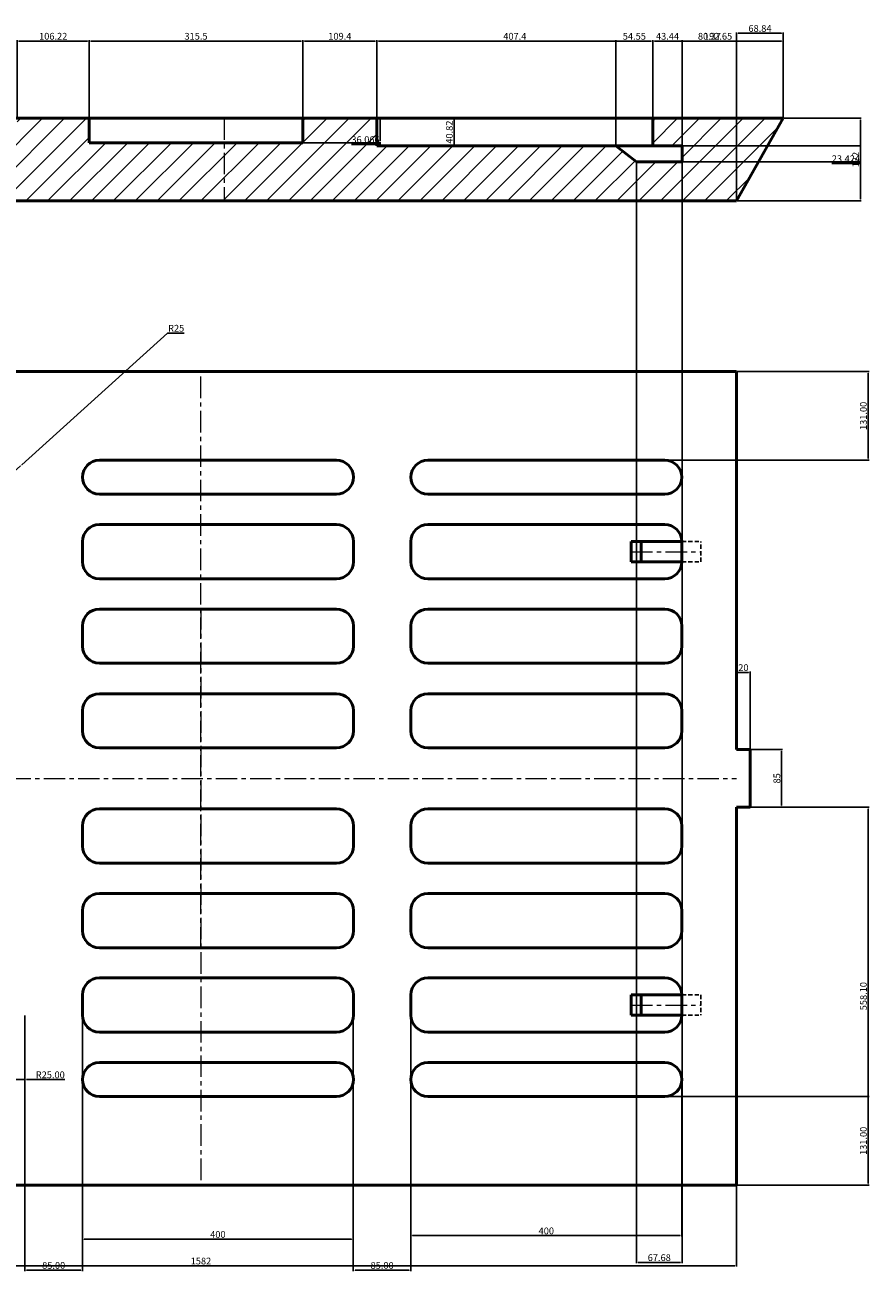
# Model space of a CAD drawing. Units: millimetres. Extents: x 1178 to 3717, y 924 to 2764.
# Tile 5 of 5: x 2471 to 3717, y 924 to 2764. Entities that reach past the tile are written whole.
import ezdxf

# ---------------------------------------------------------------- set-up
doc = ezdxf.new("R2010")
doc.units = ezdxf.units.MM
doc.linetypes.add('CENTER', pattern=[50.8, 31.75, -6.35, 6.35, -6.35])
doc.linetypes.add('HIDDEN', pattern=[9.525, 6.35, -3.175])
for name, color, linetype, lineweight in [('M-CNTR', 1, 'CENTER', 18), ('M-DIMS', 2, 'Continuous', 25), ('M-HATC', 8, 'Continuous', 18), ('M-HIDN', 6, 'HIDDEN', 25), ('M-OUTL', 7, 'Continuous', 50)]:
    doc.layers.add(name, color=color, linetype=linetype, lineweight=lineweight)
doc.styles.get("Standard").update_dxf_attribs({"font": 'arial.ttf'})
doc.dimstyles.new('ISO-25', dxfattribs={"dimtxt": 10, "dimasz": 2.5, "dimexe": 1.25, "dimexo": 0.625, "dimtad": 1, "dimtoh": 1, "dimdec": 0, "dimtxsty": 'Standard', "dimcen": 2.5, "dimadec": 0, "dimazin": 0, "dimtfac": 1, "dimtdec": 0, "dimtmove": 0, "dimatfit": 3, "dimfxl": 1, "dimarcsym": 0})

# ---------------------------------------------------------------- blocks, each defined once
blk = doc.blocks.new('*D1')
at = {"layer": 'Defpoints', "color": 0, "transparency": 16777216}
for p in [(1939.5, 1051), (3521.5, 1051), (3521.5, 932.1)]:
    blk.add_point(p, dxfattribs=at)
at = {"layer": 'M-DIMS', "color": 0, "lineweight": -2, "transparency": 16777216}
for p, q in [((1939.5, 1050.4), (1939.5, 930.9)), ((3521.5, 1050.4), (3521.5, 930.9)), ((1942, 932.1), (3519, 932.1))]:
    blk.add_line(p, q, dxfattribs=at)
at = {"layer": 'M-DIMS', "color": 0, "transparency": 16777216}
for points in [[(1942, 932.5), (1942, 931.7), (1939.5, 932.1)], [(3519, 932.5), (3519, 931.7), (3521.5, 932.1)]]:
    blk.add_solid(points, dxfattribs=at)
at = {"layer": 'M-DIMS', "color": 0, "transparency": 16777216, "insert": (2730.5, 937.8), "char_height": 10, "attachment_point": 5}
blk.add_mtext('1582', dxfattribs=at)
blk = doc.blocks.new('*D4')
at = {"layer": 'Defpoints', "color": 0, "transparency": 16777216}
for p in [(2555.5, 1207), (2955.5, 1207), (2955.5, 971.2)]:
    blk.add_point(p, dxfattribs=at)
at = {"layer": 'M-DIMS', "color": 0, "lineweight": -2, "transparency": 16777216}
for p, q in [((2555.5, 1206.4), (2555.5, 970)), ((2955.5, 1206.4), (2955.5, 970)), ((2558, 971.2), (2953, 971.2))]:
    blk.add_line(p, q, dxfattribs=at)
at = {"layer": 'M-DIMS', "color": 0, "transparency": 16777216}
for points in [[(2558, 971.7), (2558, 970.8), (2555.5, 971.2)], [(2953, 971.7), (2953, 970.8), (2955.5, 971.2)]]:
    blk.add_solid(points, dxfattribs=at)
at = {"layer": 'M-DIMS', "color": 0, "transparency": 16777216, "insert": (2755.5, 977), "char_height": 10, "attachment_point": 5}
blk.add_mtext('400', dxfattribs=at)
blk = doc.blocks.new('*D5')
at = {"layer": 'Defpoints', "color": 0, "transparency": 16777216}
for p in [(3040.5, 1207), (3440.5, 1207), (3440.5, 976.6)]:
    blk.add_point(p, dxfattribs=at)
at = {"layer": 'M-DIMS', "color": 0, "lineweight": -2, "transparency": 16777216}
for p, q in [((3040.5, 1206.4), (3040.5, 975.4)), ((3440.5, 1206.4), (3440.5, 975.4)), ((3043, 976.6), (3438, 976.6))]:
    blk.add_line(p, q, dxfattribs=at)
at = {"layer": 'M-DIMS', "color": 0, "transparency": 16777216}
for points in [[(3043, 977), (3043, 976.2), (3040.5, 976.6)], [(3438, 977), (3438, 976.2), (3440.5, 976.6)]]:
    blk.add_solid(points, dxfattribs=at)
at = {"layer": 'M-DIMS', "color": 0, "transparency": 16777216, "insert": (3240.5, 982.3), "char_height": 10, "attachment_point": 5}
blk.add_mtext('400', dxfattribs=at)
blk = doc.blocks.new('*D22')
at = {"layer": 'Defpoints', "color": 0, "transparency": 16777216}
for p in [(3541.5, 1694.1), (3541.5, 1609.1), (3587.9, 1609.1)]:
    blk.add_point(p, dxfattribs=at)
at = {"layer": 'M-DIMS', "color": 0, "lineweight": -2, "transparency": 16777216}
for p, q in [((3542.2, 1694.1), (3589.2, 1694.1)), ((3587.9, 1691.6), (3587.9, 1611.6)), ((3542.2, 1609.1), (3589.2, 1609.1))]:
    blk.add_line(p, q, dxfattribs=at)
at = {"layer": 'M-DIMS', "color": 0, "transparency": 16777216}
for points in [[(3587.5, 1691.6), (3588.3, 1691.6), (3587.9, 1694.1)], [(3587.5, 1611.6), (3588.3, 1611.6), (3587.9, 1609.1)]]:
    blk.add_solid(points, dxfattribs=at)
at = {"layer": 'M-DIMS', "color": 0, "transparency": 16777216, "insert": (3582.2, 1651.6), "char_height": 10, "attachment_point": 5, "rotation": 90}
blk.add_mtext('85', dxfattribs=at)
blk = doc.blocks.new('*D23')
at = {"layer": 'Defpoints', "color": 0, "transparency": 16777216}
for p in [(2464.1, 2113), (2445.5, 2096.2)]:
    blk.add_point(p, dxfattribs=at)
at = {"layer": 'M-DIMS', "color": 0, "lineweight": -2, "transparency": 16777216}
for p, q in [((2681.3, 2309), (2466, 2114.6)), ((2705.9, 2309), (2681.3, 2309)), ((2445.5, 2096.2), (2464.1, 2113))]:
    blk.add_line(p, q, dxfattribs=at)
at = {"layer": 'M-DIMS', "color": 0, "transparency": 16777216}
blk.add_solid([(2465.7, 2115), (2466.2, 2114.3), (2464.1, 2113)], dxfattribs=at)
at = {"layer": 'M-DIMS', "color": 0, "transparency": 16777216, "insert": (2693.9, 2314.8), "char_height": 10, "attachment_point": 5}
blk.add_mtext('R25', dxfattribs=at)
blk = doc.blocks.new('SLOT-400X80')
for p, q in [((375, 80), (25, 80)), ((0, 55), (0, 25)), ((400, 25), (400, 55)), ((25, 0), (375, 0))]:
    blk.add_line(p, q)
for centre, start, end in [((25, 55), 90, 180), ((375, 55), 0, 90), ((25, 25), 180, 270), ((375, 25), 270, 0)]:
    blk.add_arc(centre, 25, start, end)
blk = doc.blocks.new('SLOT-400X50')
for p, q in [((375, 50), (25, 50)), ((25, 0), (375, 0))]:
    blk.add_line(p, q)
for centre, start, end in [((25, 25), 90, 270), ((375, 25), 270, 90)]:
    blk.add_arc(centre, 25, start, end)
blk = doc.blocks.new('*D31')
at = {"layer": 'Defpoints', "color": 0, "transparency": 16777216}
for p in [(2565.4, 2740), (2459.2, 2626), (2565.4, 2626)]:
    blk.add_point(p, dxfattribs=at)
at = {"layer": 'M-DIMS', "color": 0, "lineweight": -2, "transparency": 16777216}
for p, q in [((2459.2, 2626.7), (2459.2, 2741.3)), ((2565.4, 2626.7), (2565.4, 2741.3)), ((2461.7, 2740), (2562.9, 2740))]:
    blk.add_line(p, q, dxfattribs=at)
at = {"layer": 'M-DIMS', "color": 0, "transparency": 16777216}
for points in [[(2461.7, 2740.5), (2461.7, 2739.6), (2459.2, 2740)], [(2562.9, 2740.5), (2562.9, 2739.6), (2565.4, 2740)]]:
    blk.add_solid(points, dxfattribs=at)
at = {"layer": 'M-DIMS', "color": 0, "transparency": 16777216, "insert": (2512.3, 2745.8), "char_height": 10, "attachment_point": 5}
blk.add_mtext('106.22', dxfattribs=at)
blk = doc.blocks.new('*D32')
at = {"layer": 'Defpoints', "color": 0, "transparency": 16777216}
for p in [(2880.9, 2740), (2565.4, 2626), (2880.9, 2626)]:
    blk.add_point(p, dxfattribs=at)
at = {"layer": 'M-DIMS', "color": 0, "lineweight": -2, "transparency": 16777216}
for p, q in [((2565.4, 2626.7), (2565.4, 2741.3)), ((2880.9, 2626.7), (2880.9, 2741.3)), ((2567.9, 2740), (2878.4, 2740))]:
    blk.add_line(p, q, dxfattribs=at)
at = {"layer": 'M-DIMS', "color": 0, "transparency": 16777216}
for points in [[(2567.9, 2740.5), (2567.9, 2739.6), (2565.4, 2740)], [(2878.4, 2740.5), (2878.4, 2739.6), (2880.9, 2740)]]:
    blk.add_solid(points, dxfattribs=at)
at = {"layer": 'M-DIMS', "color": 0, "transparency": 16777216, "insert": (2723.2, 2745.8), "char_height": 10, "attachment_point": 5}
blk.add_mtext('315.5', dxfattribs=at)
blk = doc.blocks.new('*D33')
at = {"layer": 'Defpoints', "color": 0, "transparency": 16777216}
for p in [(2990.3, 2740), (2880.9, 2626), (2990.3, 2626)]:
    blk.add_point(p, dxfattribs=at)
at = {"layer": 'M-DIMS', "color": 0, "lineweight": -2, "transparency": 16777216}
for p, q in [((2880.9, 2626.7), (2880.9, 2741.3)), ((2990.3, 2626.7), (2990.3, 2741.3)), ((2883.4, 2740), (2987.8, 2740))]:
    blk.add_line(p, q, dxfattribs=at)
at = {"layer": 'M-DIMS', "color": 0, "transparency": 16777216}
for points in [[(2883.4, 2740.5), (2883.4, 2739.6), (2880.9, 2740)], [(2987.8, 2740.5), (2987.8, 2739.6), (2990.3, 2740)]]:
    blk.add_solid(points, dxfattribs=at)
at = {"layer": 'M-DIMS', "color": 0, "transparency": 16777216, "insert": (2935.6, 2745.8), "char_height": 10, "attachment_point": 5}
blk.add_mtext('109.4', dxfattribs=at)
blk = doc.blocks.new('*D34')
at = {"layer": 'Defpoints', "color": 0, "transparency": 16777216}
for p in [(3397.7, 2740), (2990.3, 2626), (3397.7, 2626)]:
    blk.add_point(p, dxfattribs=at)
at = {"layer": 'M-DIMS', "color": 0, "lineweight": -2, "transparency": 16777216}
for p, q in [((2990.3, 2626.7), (2990.3, 2741.3)), ((3397.7, 2626.7), (3397.7, 2741.3)), ((2992.8, 2740), (3395.2, 2740))]:
    blk.add_line(p, q, dxfattribs=at)
at = {"layer": 'M-DIMS', "color": 0, "transparency": 16777216}
for points in [[(2992.8, 2740.5), (2992.8, 2739.6), (2990.3, 2740)], [(3395.2, 2740.5), (3395.2, 2739.6), (3397.7, 2740)]]:
    blk.add_solid(points, dxfattribs=at)
at = {"layer": 'M-DIMS', "color": 0, "transparency": 16777216, "insert": (3194, 2745.8), "char_height": 10, "attachment_point": 5}
blk.add_mtext('407.4', dxfattribs=at)
blk = doc.blocks.new('*D35')
at = {"layer": 'Defpoints', "color": 0, "transparency": 16777216}
for p in [(3590.4, 2740), (3397.7, 2626), (3590.4, 2626)]:
    blk.add_point(p, dxfattribs=at)
at = {"layer": 'M-DIMS', "color": 0, "lineweight": -2, "transparency": 16777216}
for p, q in [((3397.7, 2626.7), (3397.7, 2741.3)), ((3590.4, 2626.7), (3590.4, 2741.3)), ((3400.2, 2740), (3587.9, 2740))]:
    blk.add_line(p, q, dxfattribs=at)
at = {"layer": 'M-DIMS', "color": 0, "transparency": 16777216}
for points in [[(3400.2, 2740.5), (3400.2, 2739.6), (3397.7, 2740)], [(3587.9, 2740.5), (3587.9, 2739.6), (3590.4, 2740)]]:
    blk.add_solid(points, dxfattribs=at)
at = {"layer": 'M-DIMS', "color": 0, "transparency": 16777216, "insert": (3494.1, 2745.8), "char_height": 10, "attachment_point": 5}
blk.add_mtext('192.65', dxfattribs=at)
blk = doc.blocks.new('*D36')
at = {"layer": 'Defpoints', "color": 0, "transparency": 16777216}
for p in [(3590.4, 2626), (3521.5, 2504), (3704.4, 2504)]:
    blk.add_point(p, dxfattribs=at)
at = {"layer": 'M-DIMS', "color": 0, "lineweight": -2, "transparency": 16777216}
for p, q in [((3591, 2626), (3705.6, 2626)), ((3704.4, 2623.5), (3704.4, 2506.5)), ((3522.2, 2504), (3705.6, 2504))]:
    blk.add_line(p, q, dxfattribs=at)
at = {"layer": 'M-DIMS', "color": 0, "transparency": 16777216}
for points in [[(3704, 2623.5), (3704.8, 2623.5), (3704.4, 2626)], [(3704, 2506.5), (3704.8, 2506.5), (3704.4, 2504)]]:
    blk.add_solid(points, dxfattribs=at)
at = {"layer": 'M-DIMS', "color": 0, "transparency": 16777216, "insert": (3698.7, 2565), "char_height": 10, "attachment_point": 5, "rotation": 90}
blk.add_mtext('122', dxfattribs=at)
blk = doc.blocks.new('*D37')
at = {"layer": 'Defpoints', "color": 0, "transparency": 16777216}
for p in [(2880.9, 2626), (2880.9, 2590), (2994.9, 2590)]:
    blk.add_point(p, dxfattribs=at)
at = {"layer": 'M-DIMS', "color": 0, "lineweight": -2, "transparency": 16777216}
for p, q in [((2881.5, 2626), (2996.1, 2626)), ((2994.9, 2623.5), (2994.9, 2592.5)), ((2881.5, 2590), (2996.1, 2590)), ((2994.9, 2587.5), (2952.8, 2587.5)), ((2994.9, 2590), (2994.9, 2587.5))]:
    blk.add_line(p, q, dxfattribs=at)
at = {"layer": 'M-DIMS', "color": 0, "transparency": 16777216}
for points in [[(2994.5, 2623.5), (2995.3, 2623.5), (2994.9, 2626)], [(2994.5, 2592.5), (2995.3, 2592.5), (2994.9, 2590)]]:
    blk.add_solid(points, dxfattribs=at)
at = {"layer": 'M-DIMS', "color": 0, "transparency": 16777216, "insert": (2973.5, 2593.2), "char_height": 10, "attachment_point": 5}
blk.add_mtext('36.066', dxfattribs=at)
blk = doc.blocks.new('*D38')
at = {"layer": 'Defpoints', "color": 0, "transparency": 16777216}
for p in [(2990.3, 2626), (2990.3, 2585.2), (3104.3, 2585.2)]:
    blk.add_point(p, dxfattribs=at)
at = {"layer": 'M-DIMS', "color": 0, "lineweight": -2, "transparency": 16777216}
for p, q in [((2990.9, 2626), (3105.5, 2626)), ((3104.3, 2623.5), (3104.3, 2587.7)), ((2990.9, 2585.2), (3105.5, 2585.2))]:
    blk.add_line(p, q, dxfattribs=at)
at = {"layer": 'M-DIMS', "color": 0, "transparency": 16777216}
for points in [[(3103.9, 2623.5), (3104.7, 2623.5), (3104.3, 2626)], [(3103.9, 2587.7), (3104.7, 2587.7), (3104.3, 2585.2)]]:
    blk.add_solid(points, dxfattribs=at)
at = {"layer": 'M-DIMS', "color": 0, "transparency": 16777216, "insert": (3098.6, 2605.6), "char_height": 10, "attachment_point": 5, "rotation": 90}
blk.add_mtext('40.82', dxfattribs=at)
blk = doc.blocks.new('*D44')
at = {"layer": 'Defpoints', "color": 0, "transparency": 16777216}
for p in [(3397.7, 2740), (3343.2, 2585.2), (3397.7, 2585.2)]:
    blk.add_point(p, dxfattribs=at)
at = {"layer": 'M-DIMS', "color": 0, "lineweight": -2, "transparency": 16777216}
for p, q in [((3343.2, 2585.8), (3343.2, 2741.3)), ((3397.7, 2585.8), (3397.7, 2741.3)), ((3345.7, 2740), (3395.2, 2740))]:
    blk.add_line(p, q, dxfattribs=at)
at = {"layer": 'M-DIMS', "color": 0, "transparency": 16777216}
for points in [[(3345.7, 2740.5), (3345.7, 2739.6), (3343.2, 2740)], [(3395.2, 2740.5), (3395.2, 2739.6), (3397.7, 2740)]]:
    blk.add_solid(points, dxfattribs=at)
at = {"layer": 'M-DIMS', "color": 0, "transparency": 16777216, "insert": (3370.5, 2745.8), "char_height": 10, "attachment_point": 5}
blk.add_mtext('54.55', dxfattribs=at)
blk = doc.blocks.new('*D45')
at = {"layer": 'Defpoints', "color": 0, "transparency": 16777216}
for p in [(3441.2, 2740), (3397.7, 2585.2), (3441.2, 2585.2)]:
    blk.add_point(p, dxfattribs=at)
at = {"layer": 'M-DIMS', "color": 0, "lineweight": -2, "transparency": 16777216}
for p, q in [((3397.7, 2585.8), (3397.7, 2741.3)), ((3441.2, 2585.8), (3441.2, 2741.3)), ((3400.2, 2740), (3438.7, 2740))]:
    blk.add_line(p, q, dxfattribs=at)
at = {"layer": 'M-DIMS', "color": 0, "transparency": 16777216}
for points in [[(3400.2, 2740.5), (3400.2, 2739.6), (3397.7, 2740)], [(3438.7, 2740.5), (3438.7, 2739.6), (3441.2, 2740)]]:
    blk.add_solid(points, dxfattribs=at)
at = {"layer": 'M-DIMS', "color": 0, "transparency": 16777216, "insert": (3419.5, 2745.8), "char_height": 10, "attachment_point": 5}
blk.add_mtext('43.44', dxfattribs=at)
blk = doc.blocks.new('*D46')
at = {"layer": 'Defpoints', "color": 0, "transparency": 16777216}
for p in [(3521.5, 2740), (3441.2, 2585.2), (3521.5, 2504)]:
    blk.add_point(p, dxfattribs=at)
at = {"layer": 'M-DIMS', "color": 0, "lineweight": -2, "transparency": 16777216}
for p, q in [((3441.2, 2585.8), (3441.2, 2741.3)), ((3521.5, 2504.7), (3521.5, 2741.3)), ((3443.7, 2740), (3519, 2740))]:
    blk.add_line(p, q, dxfattribs=at)
at = {"layer": 'M-DIMS', "color": 0, "transparency": 16777216}
for points in [[(3443.7, 2740.5), (3443.7, 2739.6), (3441.2, 2740)], [(3519, 2740.5), (3519, 2739.6), (3521.5, 2740)]]:
    blk.add_solid(points, dxfattribs=at)
at = {"layer": 'M-DIMS', "color": 0, "transparency": 16777216, "insert": (3481.4, 2745.8), "char_height": 10, "attachment_point": 5}
blk.add_mtext('80.37', dxfattribs=at)
blk = doc.blocks.new('*D47')
at = {"layer": 'Defpoints', "color": 0, "transparency": 16777216}
for p in [(3373.5, 2561.8), (3441.2, 2561.8), (3441.2, 937)]:
    blk.add_point(p, dxfattribs=at)
at = {"layer": 'M-DIMS', "color": 0, "lineweight": -2, "transparency": 16777216}
for p, q in [((3373.5, 2561.2), (3373.5, 935.8)), ((3441.2, 2561.2), (3441.2, 935.8)), ((3376, 937), (3438.7, 937))]:
    blk.add_line(p, q, dxfattribs=at)
at = {"layer": 'M-DIMS', "color": 0, "transparency": 16777216}
for points in [[(3376, 937.4), (3376, 936.6), (3373.5, 937)], [(3438.7, 937.4), (3438.7, 936.6), (3441.2, 937)]]:
    blk.add_solid(points, dxfattribs=at)
at = {"layer": 'M-DIMS', "color": 0, "transparency": 16777216, "insert": (3407.3, 942.8), "char_height": 10, "attachment_point": 5}
blk.add_mtext('67.68', dxfattribs=at)
blk = doc.blocks.new('*D48')
at = {"layer": 'Defpoints', "color": 0, "transparency": 16777216}
for p in [(3441.2, 2585.2), (3441.2, 2561.8), (3704.4, 2561.8)]:
    blk.add_point(p, dxfattribs=at)
at = {"layer": 'M-DIMS', "color": 0, "lineweight": -2, "transparency": 16777216}
for p, q in [((3441.8, 2585.2), (3705.6, 2585.2)), ((3704.4, 2582.7), (3704.4, 2564.3)), ((3441.8, 2561.8), (3705.6, 2561.8)), ((3704.4, 2559.3), (3662.1, 2559.3)), ((3704.4, 2561.8), (3704.4, 2559.3))]:
    blk.add_line(p, q, dxfattribs=at)
at = {"layer": 'M-DIMS', "color": 0, "transparency": 16777216}
for points in [[(3704, 2582.7), (3704.8, 2582.7), (3704.4, 2585.2)], [(3704, 2564.3), (3704.8, 2564.3), (3704.4, 2561.8)]]:
    blk.add_solid(points, dxfattribs=at)
at = {"layer": 'M-DIMS', "color": 0, "transparency": 16777216, "insert": (3682.9, 2565), "char_height": 10, "attachment_point": 5}
blk.add_mtext('23.424', dxfattribs=at)
blk = doc.blocks.new('*D57')
at = {"layer": 'Defpoints', "color": 0, "transparency": 16777216}
for p in [(3541.5, 1808.1), (3521.5, 1694.1), (3541.5, 1694.1)]:
    blk.add_point(p, dxfattribs=at)
at = {"layer": 'M-DIMS', "color": 0, "lineweight": -2, "transparency": 16777216}
for p, q in [((3521.5, 1694.7), (3521.5, 1809.4)), ((3524, 1808.1), (3539, 1808.1)), ((3541.5, 1694.7), (3541.5, 1809.4))]:
    blk.add_line(p, q, dxfattribs=at)
at = {"layer": 'M-DIMS', "color": 0, "transparency": 16777216}
for points in [[(3524, 1808.5), (3524, 1807.7), (3521.5, 1808.1)], [(3539, 1808.5), (3539, 1807.7), (3541.5, 1808.1)]]:
    blk.add_solid(points, dxfattribs=at)
at = {"layer": 'M-DIMS', "color": 0, "transparency": 16777216, "insert": (3531.5, 1813.8), "char_height": 10, "attachment_point": 5}
blk.add_mtext('20', dxfattribs=at)
blk = doc.blocks.new('*D65')
at = {"layer": 'Defpoints', "color": 0, "transparency": 16777216}
for p in [(3521.5, 2751.5), (3590.4, 2626), (3521.5, 2504)]:
    blk.add_point(p, dxfattribs=at)
at = {"layer": 'M-DIMS', "color": 0, "lineweight": -2, "transparency": 16777216}
for p, q in [((3521.5, 2504.7), (3521.5, 2752.8)), ((3587.9, 2751.5), (3524, 2751.5)), ((3590.4, 2626.7), (3590.4, 2752.8))]:
    blk.add_line(p, q, dxfattribs=at)
at = {"layer": 'M-DIMS', "color": 0, "transparency": 16777216}
for points in [[(3524, 2752), (3524, 2751.1), (3521.5, 2751.5)], [(3587.9, 2752), (3587.9, 2751.1), (3590.4, 2751.5)]]:
    blk.add_solid(points, dxfattribs=at)
at = {"layer": 'M-DIMS', "color": 0, "transparency": 16777216, "insert": (3556, 2757.3), "char_height": 10, "attachment_point": 5}
blk.add_mtext('68.84', dxfattribs=at)
blk = doc.blocks.new('*D66')
at = {"layer": 'Defpoints', "color": 0, "transparency": 16777216}
for p in [(2470.5, 1302), (2555.5, 1302), (2555.5, 925.5)]:
    blk.add_point(p, dxfattribs=at)
at = {"layer": 'M-DIMS', "color": 0, "lineweight": -2, "transparency": 16777216}
for p, q in [((2470.5, 1301.4), (2470.5, 924.3)), ((2555.5, 1301.4), (2555.5, 924.3)), ((2473, 925.5), (2553, 925.5))]:
    blk.add_line(p, q, dxfattribs=at)
at = {"layer": 'M-DIMS', "color": 0, "transparency": 16777216}
for points in [[(2473, 925.9), (2473, 925.1), (2470.5, 925.5)], [(2553, 925.9), (2553, 925.1), (2555.5, 925.5)]]:
    blk.add_solid(points, dxfattribs=at)
at = {"layer": 'M-DIMS', "color": 0, "transparency": 16777216, "insert": (2513, 931.3), "char_height": 10, "attachment_point": 5}
blk.add_mtext('85.00', dxfattribs=at)
blk = doc.blocks.new('*D67')
at = {"layer": 'Defpoints', "color": 0, "transparency": 16777216}
for p in [(2955.5, 1302), (3040.5, 1302), (3040.5, 925.5)]:
    blk.add_point(p, dxfattribs=at)
at = {"layer": 'M-DIMS', "color": 0, "lineweight": -2, "transparency": 16777216}
for p, q in [((2955.5, 1301.4), (2955.5, 924.3)), ((3040.5, 1301.4), (3040.5, 924.3)), ((2958, 925.5), (3038, 925.5))]:
    blk.add_line(p, q, dxfattribs=at)
at = {"layer": 'M-DIMS', "color": 0, "transparency": 16777216}
for points in [[(2958, 925.9), (2958, 925.1), (2955.5, 925.5)], [(3038, 925.9), (3038, 925.1), (3040.5, 925.5)]]:
    blk.add_solid(points, dxfattribs=at)
at = {"layer": 'M-DIMS', "color": 0, "transparency": 16777216, "insert": (2998, 931.3), "char_height": 10, "attachment_point": 5}
blk.add_mtext('85.00', dxfattribs=at)
blk = doc.blocks.new('*D68')
at = {"layer": 'Defpoints', "color": 0, "transparency": 16777216}
for p in [(3521.5, 2252.2), (3715.9, 2252.2), (3415.5, 2121.2)]:
    blk.add_point(p, dxfattribs=at)
at = {"layer": 'M-DIMS', "color": 0, "lineweight": -2, "transparency": 16777216}
for p, q in [((3522.2, 2252.2), (3717.1, 2252.2)), ((3715.9, 2123.7), (3715.9, 2249.7)), ((3416.2, 2121.2), (3717.1, 2121.2))]:
    blk.add_line(p, q, dxfattribs=at)
at = {"layer": 'M-DIMS', "color": 0, "transparency": 16777216}
for points in [[(3715.5, 2249.7), (3716.3, 2249.7), (3715.9, 2252.2)], [(3715.5, 2123.7), (3716.3, 2123.7), (3715.9, 2121.2)]]:
    blk.add_solid(points, dxfattribs=at)
at = {"layer": 'M-DIMS', "color": 0, "transparency": 16777216, "insert": (3710.1, 2186.7), "char_height": 10, "attachment_point": 5, "rotation": 90}
blk.add_mtext('131.00', dxfattribs=at)
blk = doc.blocks.new('*D69')
at = {"layer": 'Defpoints', "color": 0, "transparency": 16777216}
for p in [(3415.5, 1182), (3521.5, 1051), (3715.9, 1051)]:
    blk.add_point(p, dxfattribs=at)
at = {"layer": 'M-DIMS', "color": 0, "lineweight": -2, "transparency": 16777216}
for p, q in [((3416.2, 1182), (3717.1, 1182)), ((3715.9, 1179.5), (3715.9, 1053.5)), ((3522.2, 1051), (3717.1, 1051))]:
    blk.add_line(p, q, dxfattribs=at)
at = {"layer": 'M-DIMS', "color": 0, "transparency": 16777216}
for points in [[(3715.5, 1179.5), (3716.3, 1179.5), (3715.9, 1182)], [(3715.5, 1053.5), (3716.3, 1053.5), (3715.9, 1051)]]:
    blk.add_solid(points, dxfattribs=at)
at = {"layer": 'M-DIMS', "color": 0, "transparency": 16777216, "insert": (3710.1, 1116.5), "char_height": 10, "attachment_point": 5, "rotation": 90}
blk.add_mtext('131.00', dxfattribs=at)
blk = doc.blocks.new('*D71')
at = {"layer": 'Defpoints', "color": 0, "transparency": 16777216}
for p in [(3541.5, 1609.1), (3715.9, 1609.1), (3521.5, 1051)]:
    blk.add_point(p, dxfattribs=at)
at = {"layer": 'M-DIMS', "color": 0, "lineweight": -2, "transparency": 16777216}
for p, q in [((3542.2, 1609.1), (3717.1, 1609.1)), ((3715.9, 1053.5), (3715.9, 1606.6)), ((3522.2, 1051), (3717.1, 1051))]:
    blk.add_line(p, q, dxfattribs=at)
at = {"layer": 'M-DIMS', "color": 0, "transparency": 16777216}
for points in [[(3715.5, 1606.6), (3716.3, 1606.6), (3715.9, 1609.1)], [(3715.5, 1053.5), (3716.3, 1053.5), (3715.9, 1051)]]:
    blk.add_solid(points, dxfattribs=at)
at = {"layer": 'M-DIMS', "color": 0, "transparency": 16777216, "insert": (3710.1, 1330.1), "char_height": 10, "attachment_point": 5, "rotation": 90}
blk.add_mtext('558.10', dxfattribs=at)
blk = doc.blocks.new('*D99')
at = {"layer": 'Defpoints', "color": 0, "transparency": 16777216}
for p in [(2445.5, 1207), (2470.5, 1207)]:
    blk.add_point(p, dxfattribs=at)
at = {"layer": 'M-DIMS', "color": 0, "lineweight": -2, "transparency": 16777216}
for p, q in [((2445.5, 1207), (2470.5, 1207)), ((2485.8, 1207), (2473, 1207)), ((2529.7, 1207), (2485.8, 1207))]:
    blk.add_line(p, q, dxfattribs=at)
at = {"layer": 'M-DIMS', "color": 0, "transparency": 16777216}
blk.add_solid([(2473, 1207.4), (2473, 1206.6), (2470.5, 1207)], dxfattribs=at)
at = {"layer": 'M-DIMS', "color": 0, "transparency": 16777216, "insert": (2508, 1212.7), "char_height": 10, "attachment_point": 5}
blk.add_mtext('R25.00', dxfattribs=at)

msp = doc.modelspace()

# ---------------------------------------------------------------- hatches: boundary and pattern name
at = {"layer": 'M-HATC'}
h = msp.add_hatch(dxfattribs=at)
h.set_pattern_fill('ANSI31', color=256, scale=7.2)
h.paths.add_polyline_path([(2053.3369, 2597.896), (2086.6296, 2597.896), (2086.6296, 2626.0416), (1939.5398, 2626.0416), (1878.7536, 2626.0416), (1939.5398, 2504.0416), (2764.9597, 2504.0416), (2764.9597, 2589.9761), (2565.4108, 2589.9761), (2565.4108, 2626.0416), (2459.1911, 2626.0416), (2459.1911, 2597.896), (2161.8062, 2597.896), (2107.2394, 2567.8003), (2053.3369, 2567.8003)])
h.paths.add_polyline_path([(3590.3795, 2626.0416), (3397.729, 2626.0416), (3397.729, 2585.2241), (3441.1717, 2585.2241), (3441.1717, 2561.8005), (3373.4902, 2561.8005), (3343.1801, 2585.2241), (2990.2894, 2585.2241), (2990.2894, 2626.0416), (2880.899, 2626.0416), (2880.899, 2589.9761), (2764.9597, 2589.9761), (2764.9597, 2504.0416), (3521.5398, 2504.0416)])

# ---------------------------------------------------------------- linework, layer by layer
at = {"layer": 'M-CNTR'}
for p, q in [((2764.9597, 2626.0416), (2764.9597, 2504.0416)), ((2730.5398, 1400.2134), (2730.5398, 2252.2134)), ((3365.7289, 1986.2134), (3468.7539, 1986.2134)), ((2730.5398, 1903.0224), (2730.5398, 1051.0224)), ((1939.5398, 1651.6179), (3521.5398, 1651.6179)), ((3365.7289, 1317.0224), (3468.7539, 1317.0224))]:
    msp.add_line(p, q, dxfattribs=at)
at = {"layer": 'M-HIDN'}
for p, q in [((3440.5398, 2001.2134), (3468.7539, 2001.2134)), ((3468.7539, 1971.2134), (3468.7539, 2001.2134)), ((3440.5398, 1971.2134), (3468.7539, 1971.2134)), ((3440.5398, 1332.0224), (3468.7539, 1332.0224)), ((3468.7539, 1332.0224), (3468.7539, 1302.0224)), ((3440.5398, 1302.0224), (3468.7539, 1302.0224))]:
    msp.add_line(p, q, dxfattribs=at)
at = {"layer": 'M-OUTL'}
for p, q in [((1939.5398, 2626.0416), (3590.3795, 2626.0416)), ((2565.4108, 2626.0416), (2565.4108, 2589.9761)), ((2880.899, 2589.9761), (2880.899, 2626.0416)), ((2990.2894, 2626.0416), (2990.2894, 2585.2241)), ((3397.729, 2585.2241), (3397.729, 2626.0416)), ((3590.3795, 2626.0416), (3521.5398, 2504.0416)), ((2565.4108, 2589.9761), (2880.899, 2589.9761)), ((2990.2894, 2585.2241), (3397.729, 2585.2241)), ((3373.4902, 2561.8005), (3343.1801, 2585.2241)), ((3397.729, 2585.2241), (3441.1717, 2585.2241)), ((3441.1717, 2585.2241), (3441.1717, 2561.8005)), ((3441.1717, 2561.8005), (3373.4902, 2561.8005)), ((3521.5398, 2504.0416), (1939.5398, 2504.0416)), ((2095.5398, 2252.2134), (3521.5398, 2252.2134)), ((3521.5398, 1903.0224), (3521.5398, 2252.2134)), ((3065.5398, 2026.2134), (3415.5398, 2026.2134)), ((3040.5398, 1971.2134), (3040.5398, 2001.2134)), ((3440.5398, 2001.2134), (3365.7289, 2001.2134)), ((3365.7289, 1971.2134), (3365.7289, 2001.2134)), ((3380.4882, 1971.2134), (3380.4882, 2001.2134)), ((3440.5398, 2001.2134), (3440.5398, 1971.2134)), ((3440.5398, 2001.2134), (3440.5398, 1971.2134)), ((3440.5398, 1971.2134), (3365.7289, 1971.2134)), ((3415.5398, 1946.2134), (3065.5398, 1946.2134)), ((3521.5398, 1694.1179), (3521.5398, 1903.0224)), ((3521.5398, 1694.1179), (3541.5398, 1694.1179)), ((3541.5398, 1694.1179), (3541.5398, 1609.1179)), ((3521.5398, 1051.0224), (3521.5398, 1609.1179)), ((3541.5398, 1609.1179), (3521.5398, 1609.1179)), ((3415.5398, 1357.0224), (3065.5398, 1357.0224)), ((3040.5398, 1332.0224), (3040.5398, 1302.0224)), ((3440.5398, 1332.0224), (3365.7289, 1332.0224)), ((3365.7289, 1332.0224), (3365.7289, 1302.0224)), ((3380.4882, 1332.0224), (3380.4882, 1302.0224)), ((3440.5398, 1302.0224), (3440.5398, 1332.0224)), ((3440.5398, 1302.0224), (3365.7289, 1302.0224)), ((3065.5398, 1277.0224), (3415.5398, 1277.0224)), ((1939.5398, 1051.0224), (3521.5398, 1051.0224))]:
    msp.add_line(p, q, dxfattribs=at)
for centre, start, end in [((3065.5398, 2001.2134), 90, 180), ((3415.5398, 2001.2134), 0, 90), ((3065.5398, 1971.2134), 180, 270), ((3415.5398, 1971.2134), 270, 0), ((3065.5398, 1332.0224), 90, 180), ((3415.5398, 1332.0224), 0, 90), ((3065.5398, 1302.0224), 180, 270), ((3415.5398, 1302.0224), 270, 0)]:
    msp.add_arc(centre, 25, start, end, dxfattribs=at)

# ---------------------------------------------------------------- block references
at = {"layer": 'M-OUTL', "rotation": 180}
for p in [(2955.5396, 2121.2139), (3440.5396, 2121.2139)]:
    msp.add_blockref('SLOT-400X50', p, dxfattribs=at)
at = {"layer": 'M-OUTL'}
for name, p in [('SLOT-400X80', (2555.54, 1946.213)), ('SLOT-400X80', (2555.54, 1821.6175)), ('SLOT-400X80', (3040.54, 1821.6175)), ('SLOT-400X80', (2555.54, 1696.6175)), ('SLOT-400X80', (3040.54, 1696.6175)), ('SLOT-400X80', (2555.54, 1526.6175)), ('SLOT-400X80', (3040.54, 1526.6175)), ('SLOT-400X80', (2555.54, 1401.6175)), ('SLOT-400X80', (3040.54, 1401.6175)), ('SLOT-400X80', (2555.54, 1277.022)), ('SLOT-400X50', (2555.54, 1182.022)), ('SLOT-400X50', (3040.54, 1182.022))]:
    msp.add_blockref(name, p, dxfattribs=at)

# ---------------------------------------------------------------- dimensions: what is measured, and where the dimension line sits
at = {"layer": 'M-DIMS'}
for base, p1, p2, override, picture, middle in [((3521.5398, 2751.5416), (3590.3795, 2626.0416), (3521.5398, 2504.0416), {"dimdec": 2, "dimlfac": 1, "dimrnd": 0, "dimzin": 0, "dimdsep": 46, "dimlunit": 2}, '*D65', (3555.9597, 2757.2723)), ((2565.4108, 2740.0416), (2459.1911, 2626.0416), (2565.4108, 2626.0416), {"dimdec": 2, "dimlfac": 1, "dimrnd": 0, "dimzin": 0, "dimdsep": 46, "dimlunit": 2}, '*D31', (2512.3009, 2745.7723)), ((2880.899, 2740.0416), (2565.4108, 2626.0416), (2880.899, 2626.0416), {"dimdec": 1, "dimlfac": 1, "dimrnd": 0, "dimzin": 0, "dimdsep": 46, "dimlunit": 2}, '*D32', (2723.1549, 2745.7757)), ((2990.2894, 2740.0416), (2880.899, 2626.0416), (2990.2894, 2626.0416), {"dimdec": 1, "dimlfac": 1, "dimrnd": 0, "dimzin": 0, "dimdsep": 46, "dimlunit": 2}, '*D33', (2935.5942, 2745.7723)), ((3397.729, 2740.0416), (2990.2894, 2626.0416), (3397.729, 2626.0416), {"dimdec": 1, "dimlfac": 1, "dimrnd": 0, "dimzin": 0, "dimdsep": 46, "dimlunit": 2}, '*D34', (3194.0092, 2745.7723)), ((3397.729, 2740.0416), (3343.1801, 2585.2241), (3397.729, 2585.2241), {"dimdec": 2, "dimlfac": 1, "dimrnd": 0, "dimzin": 0, "dimdsep": 46, "dimlunit": 2}, '*D44', (3370.4545, 2745.7518)), ((3441.1717, 2740.0416), (3397.729, 2585.2241), (3441.1717, 2585.2241), {"dimdec": 2, "dimlfac": 1, "dimrnd": 0, "dimzin": 0, "dimdsep": 46, "dimlunit": 2}, '*D45', (3419.4503, 2745.7757)), ((3590.3795, 2740.0416), (3397.729, 2626.0416), (3590.3795, 2626.0416), {"dimdec": 2, "dimlfac": 1, "dimrnd": 0, "dimzin": 0, "dimdsep": 46, "dimlunit": 2}, '*D35', (3494.0543, 2745.7723)), ((3521.5398, 2740.0416), (3441.1717, 2585.2241), (3521.5398, 2504.0416), {"dimdec": 2, "dimlfac": 1, "dimrnd": 0, "dimzin": 0, "dimdsep": 46, "dimlunit": 2}, '*D46', (3481.3558, 2745.7757)), ((3441.1717, 937.0224), (3373.4902, 2561.8005), (3441.1717, 2561.8005), {"dimdec": 2, "dimlfac": 1, "dimrnd": 0, "dimzin": 0, "dimdsep": 46, "dimlunit": 2}, '*D47', (3407.331, 942.7532)), ((3541.5398, 1808.1179), (3521.5398, 1694.1179), (3541.5398, 1694.1179), {"dimdec": 0, "dimlfac": 1, "dimrnd": 0, "dimzin": 0, "dimdsep": 46, "dimlunit": 2}, '*D57', (3531.5398, 1813.8487)), ((2555.5398, 925.5224), (2470.5398, 1302.0224), (2555.5398, 1302.0224), {"dimdec": 2, "dimlfac": 1, "dimrnd": 0, "dimzin": 0, "dimdsep": 46, "dimlunit": 2}, '*D66', (2513.0398, 931.2532)), ((3040.5398, 925.5224), (2955.5398, 1302.0224), (3040.5398, 1302.0224), {"dimdec": 2, "dimlfac": 1, "dimrnd": 0, "dimzin": 0, "dimdsep": 46, "dimlunit": 2}, '*D67', (2998.0398, 931.2532)), ((2955.5398, 971.239), (2555.5398, 1207.0224), (2955.5398, 1207.0224), {"dimclrd": 0, "dimclre": 0, "dimclrt": 0}, '*D4', (2755.5398, 976.9697)), ((3440.5398, 976.6022), (3040.5398, 1207.0224), (3440.5398, 1207.0224), {"dimclrd": 0, "dimclre": 0, "dimclrt": 0}, '*D5', (3240.5398, 982.3329)), ((3521.5398, 932.1144), (1939.5398, 1051.0224), (3521.5398, 1051.0224), {"dimclrd": 0, "dimclre": 0, "dimclrt": 0}, '*D1', (2730.5398, 937.8451))]:
    dim = msp.add_linear_dim(base=base, p1=p1, p2=p2, dimstyle='ISO-25', override=override, dxfattribs=at)
    dim.commit()
    dim.dimension.update_dxf_attribs({"geometry": picture, "text_midpoint": middle})
for base, p1, p2, angle, override, picture, middle in [((2994.899007, 2589.976075), (2880.899007, 2626.041582), (2880.899007, 2589.976075), 270, {"dimdec": 3, "dimlfac": 1, "dimrnd": 0, "dimzin": 0, "dimdsep": 46, "dimlunit": 2}, '*D37', (2973.523666, 2593.210216)), ((3104.2894, 2585.2241), (2990.2894, 2626.0416), (2990.2894, 2585.2241), 270, {"dimdec": 2, "dimlfac": 1, "dimrnd": 0, "dimzin": 0, "dimdsep": 46, "dimlunit": 2}, '*D38', (3098.5587, 2605.6329)), ((3704.3796, 2504.0416), (3590.3795, 2626.0416), (3521.5398, 2504.0416), 90, {"dimdec": 0, "dimlfac": 1, "dimrnd": 0, "dimzin": 0, "dimdsep": 46, "dimlunit": 2}, '*D36', (3698.7341, 2565.0416)), ((3704.3796, 2561.8005), (3441.1717, 2585.2241), (3441.1717, 2561.8005), 90, {"dimdec": 3, "dimlfac": 1, "dimrnd": 0, "dimzin": 0, "dimdsep": 46, "dimlunit": 2}, '*D48', (3682.9326, 2565.0347)), ((3715.8796, 2252.2134), (3415.5398, 2121.2134), (3521.5398, 2252.2134), 90, {"dimdec": 2, "dimlfac": 1, "dimrnd": 0, "dimzin": 0, "dimdsep": 46, "dimlunit": 2}, '*D68', (3710.1454, 2186.7134)), ((3587.9286, 1609.1179), (3541.5398, 1694.1179), (3541.5398, 1609.1179), 90, {"dimclrd": 0, "dimclre": 0, "dimclrt": 0}, '*D22', (3582.1979, 1651.6179)), ((3715.8796, 1609.1179), (3521.5398, 1051.0224), (3541.5398, 1609.1179), 90, {"dimdec": 2, "dimlfac": 1, "dimrnd": 0, "dimzin": 0, "dimdsep": 46, "dimlunit": 2}, '*D71', (3710.1488, 1330.0702)), ((3715.8796, 1051.0224), (3415.5398, 1182.0224), (3521.5398, 1051.0224), 90, {"dimdec": 2, "dimlfac": 1, "dimrnd": 0, "dimzin": 0, "dimdsep": 46, "dimlunit": 2}, '*D69', (3710.1454, 1116.5224))]:
    dim = msp.add_linear_dim(base=base, p1=p1, p2=p2, angle=angle, dimstyle='ISO-25', override=override, dxfattribs=at)
    dim.commit()
    dim.dimension.update_dxf_attribs({"geometry": picture, "text_midpoint": middle})
dim = msp.add_radius_dim(center=(2445.5398, 2096.2134), mpoint=(2464.0957, 2112.9669), dimstyle='ISO-25', override={"dimclrd": 0, "dimclre": 0, "dimclrt": 0}, dxfattribs=at)
dim.commit()
dim.dimension.update_dxf_attribs({"geometry": '*D23', "text_midpoint": (2693.8758, 2309.0425), "dimtype": 164})
dim = msp.add_radius_dim(center=(2445.5398, 1207.0224), mpoint=(2470.5398, 1207.02), dimstyle='ISO-25', override={"dimdec": 2, "dimlfac": 1, "dimrnd": 0, "dimzin": 0, "dimdsep": 46, "dimlunit": 2}, dxfattribs=at)
dim.commit()
dim.dimension.update_dxf_attribs({"geometry": '*D99', "text_midpoint": (2508.0168, 1212.7492)})

doc.saveas('drawing.dxf')
